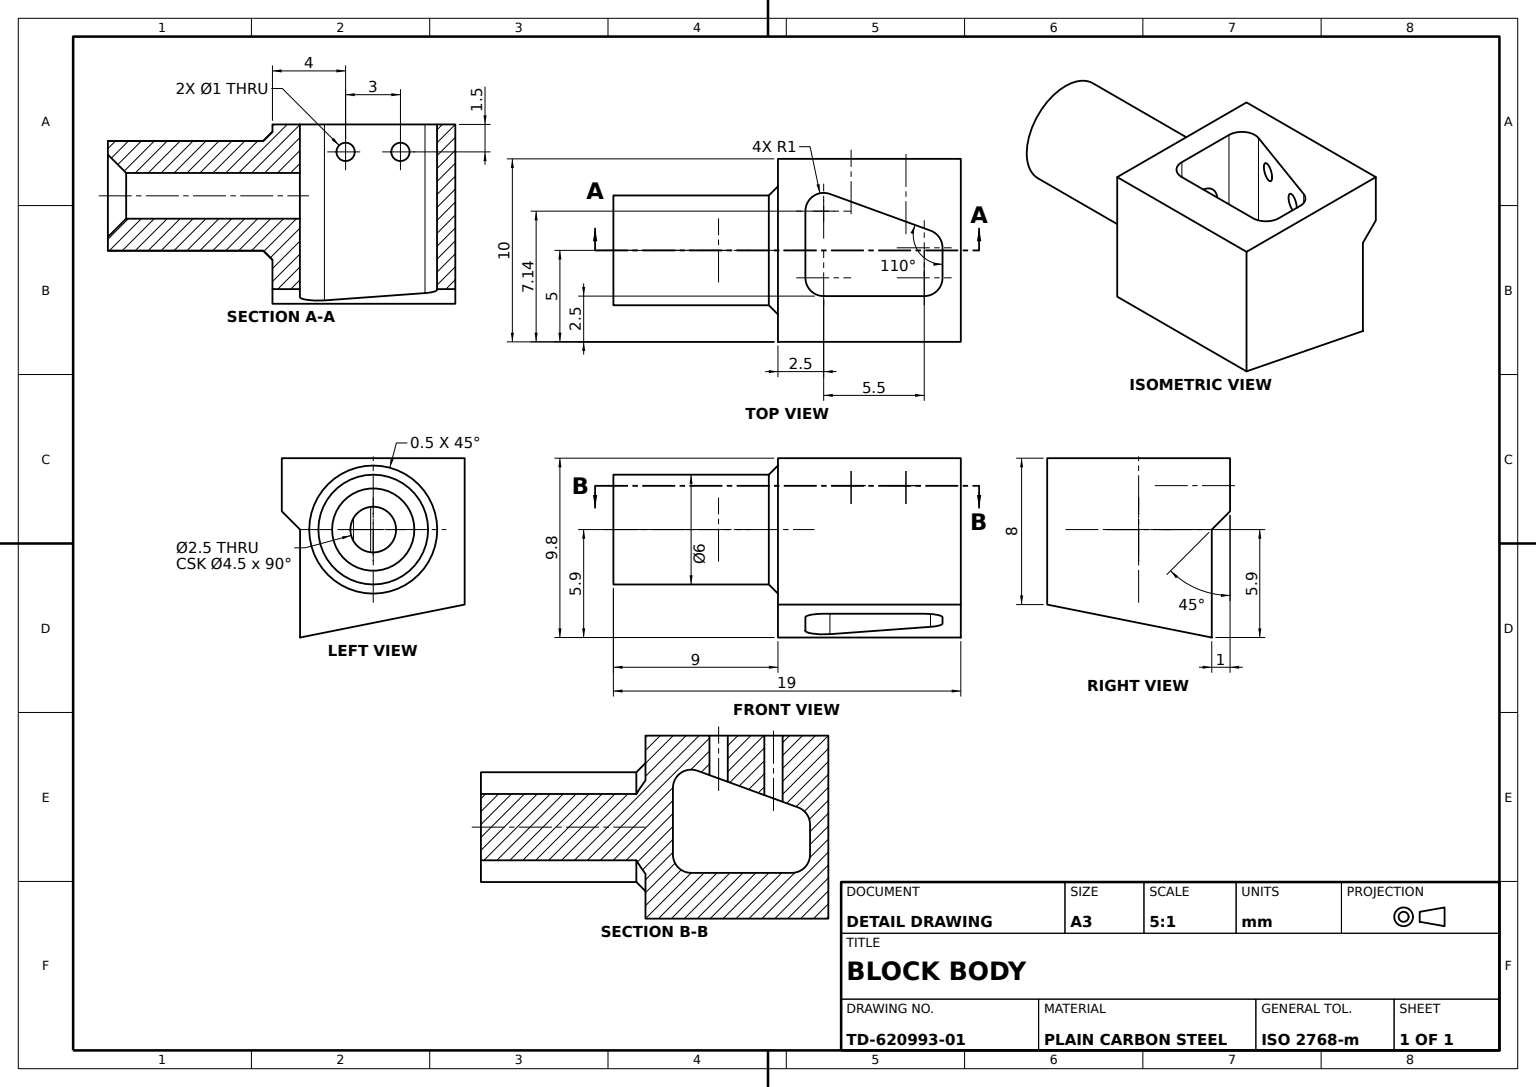
SolidWorks part; units mm, degrees
material "Plain Carbon Steel"
ref_plane "Front Plane" through (0, 0, 0) normal (0, 0, 1) x (1, 0, 0)
ref_plane "Top Plane" through (0, 0, 0) normal (0, 1, 0) x (1, 0, 0)
ref_plane "Right Plane" through (0, 0, 0) normal (1, 0, 0) x (0, 0, -1)
sketch "Base Block Sketch" plane through (0, 0, 0) normal (0, 0, 1) x (1, 0, 0)
  line L0 (0, 0) -> (10, 0)
  line L1 (10, 0) -> (10, -8)
  line L2 (0, 0) -> (0, -10)
  line L3 (0, -10) -> (10, -8)
  dimension "D1" = 10
  dimension "D2" = 8
  dimension "D3" = 10
extrude "Base Block" add sketch "Base Block Sketch" along normal blind 10
sketch "Spigot Sketch" plane through (0, 0, 10) normal (0, 0, 1) x (1, 0, 0)
  line L0 (0, -10) -> (10, -8)
  line L1 (10, 0) -> (5, 0)
  line L3 (10, 0) -> (0, 0) construction
  line L5 (5, 0) -> (5, -9)
  line L6 (5.9378, -8.8124) -> (5, -3.9012)
  circle A0 centre (5, -3.9012) radius 3
  dimension "D3" = 6
  dimension "D1" = 5
  dimension "D2" = 5
  dimension "D4" = 4.9998
extrude "Round Spigot" add sketch "Spigot Sketch" along normal blind 9 contours L5 A0 | L6 A0 L5 | L5 A0 L6
sketch "Profile Cut A Sketch" plane through (0, 0, 10) normal (0, 0, 1) x (1, 0, 0)
  line L3 (0, 0) -> (0, -2.9012)
  line L6 (1, -3.9012) -> (0, -2.9012)
  line L7 (1, -3.9012) -> (1, -9.8)
  line L8 (0, -2.9012) -> (0, -10)
  line L9 (0, -10) -> (1, -9.8)
  line L10 (0, -10) -> (10, -8) construction
  line M6 (0, 0) -> (0, -10)
  line M7 (0, -10) -> (10, -8)
  dimension "D1" = 5.8988
  dimension "D2" = 1
  dimension "D3" = 1.4142
extrude "Profile Cut A" cut sketch "Profile Cut A Sketch" against normal blind 10 contours L7 L6 M6 M7
sketch "Triangular Pocket Sketch" plane through (0, 0, 0) normal (0, 1, 0) x (1, 0, 0)
  line L0 (10, -10) -> (10, 0) construction
  line L2 (10, -10) -> (0, -10) construction
  line L4 (2.6508, -5.1449) -> (3.9199, -1.658)
  line L5 (0, -10) -> (0, 0) construction
  line L6 (2.6508, -5.1449) -> (1.9181, -7.158)
  line L7 (5, -8.5) -> (6.5, -8.5)
  line L8 (7.5, -7.5) -> (7.5, -2)
  line L9 (6.5, -1) -> (4.8596, -1)
  line L10 (5, -8.5) -> (2.8578, -8.5)
  circle A0 centre (5, -6) radius 2.5 construction
  arc A1 (6.5, -8.5) -> (7.5, -7.5) centre (6.5, -7.5) ccw
  arc A2 (7.5, -2) -> (6.5, -1) centre (6.5, -2) ccw
  arc A3 (4.8596, -1) -> (3.9199, -1.658) centre (4.8596, -2) ccw
  arc A4 (2.8578, -8.5) -> (1.9181, -7.158) centre (2.8578, -7.5) cw
  dimension "D2" = 5
  dimension "D1" = 1
  dimension "D3" = 5.5
  dimension "D4" = 20
  dimension "D5" = 3.7108
  dimension "D6" = 5
  dimension "D7" = 1.5
extrude "Triangular Pocket" cut sketch "Triangular Pocket Sketch" against normal blind 10
sketch "Profile Cut B Sketch" plane through (0, 0, 0) normal (-1, 0, 0) x (0, 0, 1)
  line L0 (10, 0) -> (10, -1.5)
  line L1 (10, -6.9012) -> (10, -0.9012) construction
  line L2 (10, -1.5) -> (6, -1.5)
  line L3 (6, -1.5) -> (3, -1.5)
  circle A0 centre (3, -1.5) radius 0.5
  circle A1 centre (6, -1.5) radius 0.5
  dimension "D4" = 1
  dimension "D5" = 1
  dimension "D1" = 1.5
  dimension "D2" = 4
  dimension "D3" = 3
extrude "Profile Cut B" cut sketch "Profile Cut B Sketch" against normal blind 5
chamfer "Spigot Chamfer 0.5" distance 0.5 angle 45 1 edges at (8, -3.9012, 10)
sketch "Spigot Bore Sketch" plane through (0, 0, 19) normal (0, 0, 1) x (1, 0, 0)
  circle A0 centre (5, -3.9012) radius 1.25
  dimension "D1" = 2.5
extrude "Spigot Bore" cut sketch "Spigot Bore Sketch" against normal blind 12
chamfer "Bore Chamfer 1" distance 1 angle 45 1 edges at (6.25, -3.9012, 19)
